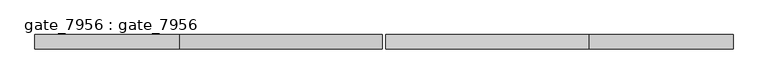
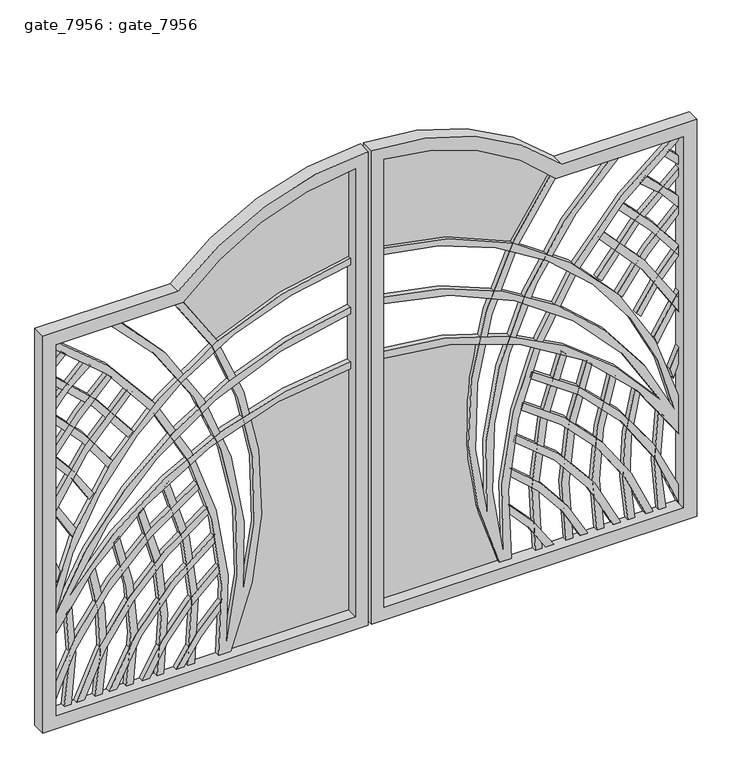
"""IFC4 building model written with IfcOpenShell, lengths in millimetres: proxy geometry, gate_7956 : gate_7956."""

from ifc_helpers import new_model, si_unit, point, frame, frame_2d, origin, place, context, project, spatial, polyline, circle_curve, trimmed, segment, composite_curve, outline, extrude, source, transform, mapped, element, save


def gate_7956_gate_7956_6bc30956(model_context):
    return source(origin(), model_context, "Body", "SweptSolid", [
        extrude(outline(composite_curve([segment(polyline([(1574.8, -714.375), (1574.8, -1222.375), (0.0, -1222.375), (0.0, 0.0), (1879.3736556, 0.0)]), True, "CONTINUOUS"), segment(trimmed(circle_curve(frame_2d((881.859553, 3.175)), 997.5191555), [point((1879.3736556, 0.0))], [point((1574.8, -714.375))], False, "CARTESIAN"), True, "CONTINUOUS")], self_intersect=False), holes=[composite_curve([segment(polyline([(1827.2147875, -47.625), (50.8, -47.625), (50.8, -1171.575), (1524.0, -1171.575), (1524.0, -692.4777911)]), True, "CONTINUOUS"), segment(trimmed(circle_curve(frame_2d((881.859553, 3.175)), 946.7191555), [point((1524.0, -692.4777911))], [point((1827.2147875, -47.625))], True, "CARTESIAN"), True, "CONTINUOUS")], self_intersect=False)]), frame((0.0, -50.8, 0.0), z_axis=(0.0, 1.0, 0.0), x_axis=(0.0, 0.0, 1.0)), (0.0, 0.0, 1.0), 50.8),
        extrude(outline(composite_curve([segment(trimmed(circle_curve(frame_2d((188.1193765, 65.6258097)), 1270.1981582), [point((1453.2587424, -47.625))], [point((475.7606767, -1171.575))], False, "CARTESIAN"), True, "CONTINUOUS"), segment(polyline([(475.7606767, -1171.575), (325.438753, -1171.575)]), True, "CONTINUOUS"), segment(trimmed(circle_curve(frame_2d((-306.470048, -9.2092819)), 1323.0278891), [point((325.438753, -1171.575))], [point((1016.0, -47.625))], True, "CARTESIAN"), True, "CONTINUOUS"), segment(polyline([(1016.0, -47.625), (1042.85139, -47.625)]), True, "CONTINUOUS"), segment(trimmed(circle_curve(frame_2d((-321.9912288, -1.7370637)), 1365.6138095), [point((1042.85139, -47.625))], [point((487.9033995, -1101.269586))], False, "CARTESIAN"), True, "CONTINUOUS"), segment(trimmed(circle_curve(frame_2d((-94.5667128, 101.7568292)), 1336.6166195), [point((487.9033995, -1101.269586))], [point((1233.6761327, -47.625))], True, "CARTESIAN"), True, "CONTINUOUS"), segment(polyline([(1233.6761327, -47.625), (1259.2332506, -47.625)]), True, "CONTINUOUS"), segment(trimmed(circle_curve(frame_2d((-94.5667128, 101.7568292)), 1362.0166195), [point((1259.2332506, -47.625))], [point((428.8390935, -1155.6753295))], False, "CARTESIAN"), True, "CONTINUOUS"), segment(trimmed(circle_curve(frame_2d((188.1193765, 65.6258097)), 1244.7981582), [point((428.8390935, -1155.6753295))], [point((1427.7550927, -47.625))], True, "CARTESIAN"), True, "CONTINUOUS"), segment(polyline([(1427.7550927, -47.625), (1453.2587424, -47.625)]), True, "CONTINUOUS")], self_intersect=False)), frame((0.0, -19.05, 0.0), z_axis=(0.0, 1.0, 0.0), x_axis=(0.0, 0.0, 1.0)), (0.0, 0.0, 1.0), 19.05),
        extrude(outline(composite_curve([segment(trimmed(circle_curve(frame_2d((625.1927136, -1831.8247988)), 1451.1947292), [point((50.8, -499.1436094))], [point((1524.0, -692.4777911))], False, "CARTESIAN"), True, "CONTINUOUS"), segment(polyline([(1524.0, -692.4777911), (1524.0, -717.8616311), (1508.2761961, -712.4096154)]), True, "CONTINUOUS"), segment(trimmed(circle_curve(frame_2d((625.2005352, -1831.8604357)), 1425.8305516), [point((1508.2761961, -712.4096154))], [point((270.5135839, -450.849962))], True, "CARTESIAN"), True, "CONTINUOUS"), segment(trimmed(circle_curve(frame_2d((428.9211986, -1911.4736244)), 1469.1883662), [point((270.5135839, -450.849962))], [point((1524.0, -932.0263955))], False, "CARTESIAN"), True, "CONTINUOUS"), segment(polyline([(1524.0, -932.0263955), (1524.0, -970.5462776)]), True, "CONTINUOUS"), segment(trimmed(circle_curve(frame_2d((434.6192112, -1905.6521568)), 1435.6787622), [point((1524.0, -970.5462776))], [point((79.5169904, -514.5820935))], True, "CARTESIAN"), True, "CONTINUOUS"), segment(trimmed(circle_curve(frame_2d((251.9754674, -2051.8469137)), 1546.9082241), [point((79.5169904, -514.5820935))], [point((1524.0, -1171.575))], False, "CARTESIAN"), True, "CONTINUOUS"), segment(polyline([(1524.0, -1171.575), (1492.986601, -1171.575)]), True, "CONTINUOUS"), segment(trimmed(circle_curve(frame_2d((251.9754674, -2051.8469137)), 1521.5082241), [point((1492.986601, -1171.575))], [point((50.8, -543.6971508))], True, "CARTESIAN"), True, "CONTINUOUS"), segment(polyline([(50.8, -543.6971508), (50.8, -499.1436094)]), True, "CONTINUOUS")], self_intersect=False)), frame((0.0, -19.05, 0.0), z_axis=(0.0, 1.0, 0.0), x_axis=(0.0, 0.0, 1.0)), (0.0, 0.0, 1.0), 19.05),
        extrude(outline(composite_curve([segment(trimmed(circle_curve(frame_2d((-321.9912288, -1.7370636)), 1251.3138095), [point((766.023996, -619.8059275))], [point((122.1545272, -1171.575))], False, "CARTESIAN"), True, "CONTINUOUS"), segment(polyline([(122.1545272, -1171.575), (50.8, -1171.575)]), True, "CONTINUOUS"), segment(trimmed(circle_curve(frame_2d((-329.3476454, 3.2021804)), 1234.7524675), [point((50.8, -1171.575))], [point((741.6413557, -611.2864))], True, "CARTESIAN"), True, "CONTINUOUS"), segment(polyline([(741.6413557, -611.2864), (766.023996, -619.8059275)]), True, "CONTINUOUS")], self_intersect=False)), frame((0.0, -19.05, 0.0), z_axis=(0.0, 1.0, 0.0), x_axis=(0.0, 0.0, 1.0)), (0.0, 0.0, 1.0), 19.05),
        extrude(outline(composite_curve([segment(trimmed(circle_curve(frame_2d((-321.9912288, -1.7370637)), 1137.0138095), [point((654.3216834, -584.5007383))], [point((50.8, -1075.9005069))], False, "CARTESIAN"), True, "CONTINUOUS"), segment(polyline([(50.8, -1075.9005069), (50.8, -1048.9772277)]), True, "CONTINUOUS"), segment(trimmed(circle_curve(frame_2d((-321.9912288, -1.7370637)), 1111.6138095), [point((50.8, -1048.9772277))], [point((628.7552213, -577.7287729))], True, "CARTESIAN"), True, "CONTINUOUS"), segment(polyline([(628.7552213, -577.7287729), (654.3216834, -584.5007383)]), True, "CONTINUOUS")], self_intersect=False)), frame((0.0, -19.05, 0.0), z_axis=(0.0, 1.0, 0.0), x_axis=(0.0, 0.0, 1.0)), (0.0, 0.0, 1.0), 19.05),
        extrude(outline(composite_curve([segment(trimmed(circle_curve(frame_2d((-321.9912288, -1.7370637)), 1022.7138095), [point((536.7182406, -557.2202617))], [point((50.8, -954.0869132))], False, "CARTESIAN"), True, "CONTINUOUS"), segment(polyline([(50.8, -954.0869132), (50.8, -926.7568118)]), True, "CONTINUOUS"), segment(trimmed(circle_curve(frame_2d((-321.9912288, -1.7370637)), 997.3138095), [point((50.8, -926.7568118))], [point((510.8571668, -550.3702604))], True, "CARTESIAN"), True, "CONTINUOUS"), segment(polyline([(510.8571668, -550.3702604), (536.7182406, -557.2202617)]), True, "CONTINUOUS")], self_intersect=False)), frame((0.0, -19.05, 0.0), z_axis=(0.0, 1.0, 0.0), x_axis=(0.0, 0.0, 1.0)), (0.0, 0.0, 1.0), 19.05),
        extrude(outline(composite_curve([segment(trimmed(circle_curve(frame_2d((-321.9912288, -1.7370637)), 908.4138095), [point((410.7722159, -538.6480277))], [point((50.8, -830.134522))], False, "CARTESIAN"), True, "CONTINUOUS"), segment(polyline([(50.8, -830.134522), (50.8, -802.1994847)]), True, "CONTINUOUS"), segment(trimmed(circle_curve(frame_2d((-321.9912288, -1.7370637)), 883.0138095), [point((50.8, -802.1994847))], [point((379.0365912, -538.6480277))], True, "CARTESIAN"), True, "CONTINUOUS"), segment(polyline([(379.0365912, -538.6480277), (410.7722159, -538.6480277)]), True, "CONTINUOUS")], self_intersect=False)), frame((0.0, -19.05, 0.0), z_axis=(0.0, 1.0, 0.0), x_axis=(0.0, 0.0, 1.0)), (0.0, 0.0, 1.0), 19.05),
        extrude(outline(composite_curve([segment(trimmed(circle_curve(frame_2d((-321.9912288, -1.7370637)), 794.1138095), [point((270.5266887, -530.4517881))], [point((50.8, -702.9099683))], False, "CARTESIAN"), True, "CONTINUOUS"), segment(polyline([(50.8, -702.9099683), (50.8, -674.0075603)]), True, "CONTINUOUS"), segment(trimmed(circle_curve(frame_2d((-321.9912288, -1.7370637)), 768.7138095), [point((50.8, -674.0075603))], [point((236.0245963, -530.4517881))], True, "CARTESIAN"), True, "CONTINUOUS"), segment(polyline([(236.0245963, -530.4517881), (270.5266887, -530.4517881)]), True, "CONTINUOUS")], self_intersect=False)), frame((0.0, -19.05, 0.0), z_axis=(0.0, 1.0, 0.0), x_axis=(0.0, 0.0, 1.0)), (0.0, 0.0, 1.0), 19.05),
        extrude(outline(composite_curve([segment(polyline([(1210.9602193, -867.4506933), (1228.939295, -885.429769)]), True, "CONTINUOUS"), segment(trimmed(circle_curve(frame_2d((188.1193765, 65.6258097)), 1409.8981582), [point((1228.939295, -885.429769))], [point((864.245824, -1171.575))], False, "CARTESIAN"), True, "CONTINUOUS"), segment(polyline([(864.245824, -1171.575), (809.5445985, -1171.575)]), True, "CONTINUOUS"), segment(trimmed(circle_curve(frame_2d((188.1193765, 65.6258097)), 1384.4981582), [point((809.5445985, -1171.575))], [point((1210.9602193, -867.4506933))], True, "CARTESIAN"), True, "CONTINUOUS")], self_intersect=False)), frame((0.0, -19.05, 0.0), z_axis=(0.0, 1.0, 0.0), x_axis=(0.0, 0.0, 1.0)), (0.0, 0.0, 1.0), 19.05),
        extrude(outline(composite_curve([segment(polyline([(1295.7670706, -944.0833092), (1313.7464656, -962.0627043)]), True, "CONTINUOUS"), segment(trimmed(circle_curve(frame_2d((298.9547736, -40.580869)), 1370.7410225), [point((1313.7464656, -962.0627043))], [point((1073.4115036, -1171.575))], False, "CARTESIAN"), True, "CONTINUOUS"), segment(polyline([(1073.4115036, -1171.575), (1034.1276953, -1171.575)]), True, "CONTINUOUS"), segment(trimmed(circle_curve(frame_2d((188.1193765, 65.6258097)), 1498.7981582), [point((1034.1276953, -1171.575))], [point((1295.7670706, -944.0833092))], True, "CARTESIAN"), True, "CONTINUOUS")], self_intersect=False)), frame((0.0, -19.05, 0.0), z_axis=(0.0, 1.0, 0.0), x_axis=(0.0, 0.0, 1.0)), (0.0, 0.0, 1.0), 19.05),
        extrude(outline(composite_curve([segment(polyline([(1371.3808408, -1023.8325474), (1393.8084123, -1046.2601189)]), True, "CONTINUOUS"), segment(trimmed(circle_curve(frame_2d((157.0059526, 65.2274597)), 1662.854462), [point((1393.8084123, -1046.2601189))], [point((1268.4935312, -1171.575))], False, "CARTESIAN"), True, "CONTINUOUS"), segment(polyline([(1268.4935312, -1171.575), (1223.2134903, -1171.575)]), True, "CONTINUOUS"), segment(trimmed(circle_curve(frame_2d((881.0604584, -680.2699964)), 598.7063586), [point((1223.2134903, -1171.575))], [point((1371.3808408, -1023.8325474))], True, "CARTESIAN"), True, "CONTINUOUS")], self_intersect=False)), frame((0.0, -19.05, 0.0), z_axis=(0.0, 1.0, 0.0), x_axis=(0.0, 0.0, 1.0)), (0.0, 0.0, 1.0), 19.05),
        extrude(outline(composite_curve([segment(polyline([(1448.1437026, -1116.942791), (1466.2607278, -1135.0598162)]), True, "CONTINUOUS"), segment(trimmed(circle_curve(frame_2d((2369.5144168, -2074.828689)), 1303.469509), [point((1466.2607278, -1135.0598162))], [point((1429.745544, -1171.575))], True, "CARTESIAN"), True, "CONTINUOUS"), segment(polyline([(1429.745544, -1171.575), (1393.6228205, -1171.575)]), True, "CONTINUOUS"), segment(trimmed(circle_curve(frame_2d((2581.8039176, -2302.8138821)), 1640.5717686), [point((1393.6228205, -1171.575))], [point((1448.1437026, -1116.942791))], False, "CARTESIAN"), True, "CONTINUOUS")], self_intersect=False)), frame((0.0, -19.05, 0.0), z_axis=(0.0, 1.0, 0.0), x_axis=(0.0, 0.0, 1.0)), (0.0, 0.0, 1.0), 19.05),
        extrude(outline(composite_curve([segment(polyline([(50.8, -1123.3836365), (50.8, -1096.2682984)]), True, "CONTINUOUS"), segment(trimmed(circle_curve(frame_2d((249.227799, -2294.693819)), 1214.741668), [point((50.8, -1096.2682984))], [point((439.2593722, -1094.9082877))], False, "CARTESIAN"), True, "CONTINUOUS"), segment(polyline([(439.2593722, -1094.9082877), (417.7529701, -1116.4146899)]), True, "CONTINUOUS"), segment(trimmed(circle_curve(frame_2d((251.9754674, -2051.8469137)), 950.0082241), [point((417.7529701, -1116.4146899))], [point((50.8, -1123.3836365))], True, "CARTESIAN"), True, "CONTINUOUS")], self_intersect=False)), frame((0.0, -19.05, 0.0), z_axis=(0.0, 1.0, 0.0), x_axis=(0.0, 0.0, 1.0)), (0.0, 0.0, 1.0), 19.05),
        extrude(outline(composite_curve([segment(polyline([(50.8, -1006.7247069), (50.8, -980.869582)]), True, "CONTINUOUS"), segment(trimmed(circle_curve(frame_2d((251.9754674, -2051.8469137)), 1089.7082241), [point((50.8, -980.869582))], [point((559.4182819, -1006.4078053))], False, "CARTESIAN"), True, "CONTINUOUS"), segment(polyline([(559.4182819, -1006.4078053), (538.8861292, -1026.939958)]), True, "CONTINUOUS"), segment(trimmed(circle_curve(frame_2d((251.9754674, -2051.8469137)), 1064.3082241), [point((538.8861292, -1026.939958))], [point((50.8, -1006.7247069))], True, "CARTESIAN"), True, "CONTINUOUS")], self_intersect=False)), frame((0.0, -19.05, 0.0), z_axis=(0.0, 1.0, 0.0), x_axis=(0.0, 0.0, 1.0)), (0.0, 0.0, 1.0), 19.05),
        extrude(outline(composite_curve([segment(polyline([(50.8, -890.30598), (50.8, -864.7646777)]), True, "CONTINUOUS"), segment(trimmed(circle_curve(frame_2d((251.9754674, -2051.8469137)), 1204.0082241), [point((50.8, -864.7646777))], [point((656.0575932, -917.6716895))], False, "CARTESIAN"), True, "CONTINUOUS"), segment(polyline([(656.0575932, -917.6716895), (636.1282841, -937.6009986)]), True, "CONTINUOUS"), segment(trimmed(circle_curve(frame_2d((249.671635, -2074.7397377)), 1201.0134277), [point((636.1282841, -937.6009986))], [point((50.8, -890.30598))], True, "CARTESIAN"), True, "CONTINUOUS")], self_intersect=False)), frame((0.0, -19.05, 0.0), z_axis=(0.0, 1.0, 0.0), x_axis=(0.0, 0.0, 1.0)), (0.0, 0.0, 1.0), 19.05),
        extrude(outline(composite_curve([segment(polyline([(50.8, -774.6859578), (50.8, -748.9789216)]), True, "CONTINUOUS"), segment(trimmed(circle_curve(frame_2d((251.9754674, -2051.8469137)), 1318.3082241), [point((50.8, -748.9789216))], [point((737.9350335, -826.3756274))], False, "CARTESIAN"), True, "CONTINUOUS"), segment(polyline([(737.9350335, -826.3756274), (718.3335001, -845.9771607)]), True, "CONTINUOUS"), segment(trimmed(circle_curve(frame_2d((251.9754674, -2051.8469137)), 1292.9082241), [point((718.3335001, -845.9771607))], [point((50.8, -774.6859578))], True, "CARTESIAN"), True, "CONTINUOUS")], self_intersect=False)), frame((0.0, -19.05, 0.0), z_axis=(0.0, 1.0, 0.0), x_axis=(0.0, 0.0, 1.0)), (0.0, 0.0, 1.0), 19.05),
        extrude(outline(composite_curve([segment(polyline([(50.8, -659.0930168), (50.8, -633.4341547)]), True, "CONTINUOUS"), segment(trimmed(circle_curve(frame_2d((251.9754674, -2051.8469137)), 1432.6082241), [point((50.8, -633.4341547))], [point((808.380048, -731.7028813))], False, "CARTESIAN"), True, "CONTINUOUS"), segment(polyline([(808.380048, -731.7028813), (788.9599222, -751.1230071)]), True, "CONTINUOUS"), segment(trimmed(circle_curve(frame_2d((251.9754674, -2051.8469137)), 1407.2082241), [point((788.9599222, -751.1230071))], [point((50.8, -659.0930168))], True, "CARTESIAN"), True, "CONTINUOUS")], self_intersect=False)), frame((0.0, -19.05, 0.0), z_axis=(0.0, 1.0, 0.0), x_axis=(0.0, 0.0, 1.0)), (0.0, 0.0, 1.0), 19.05),
        extrude(outline(polyline([(553.3842288, -1150.9205103), (593.450224, -1138.1641492), (672.1451492, -1171.575), (609.2386529, -1171.575), (553.3842288, -1150.9205103)])), frame((0.0, -19.05, 0.0), z_axis=(0.0, 1.0, 0.0), x_axis=(0.0, 0.0, 1.0)), (0.0, 0.0, 1.0), 19.05),
        extrude(outline(composite_curve([segment(trimmed(circle_curve(frame_2d((251.9754673, -2051.8469137)), 1064.3082241), [point((850.2006371, -1171.575))], [point((711.3700205, -1091.7903318))], True, "CARTESIAN"), True, "CONTINUOUS"), segment(polyline([(711.3700205, -1091.7903318), (740.9012216, -1077.980588)]), True, "CONTINUOUS"), segment(trimmed(circle_curve(frame_2d((251.9754674, -2051.8469137)), 1089.7082241), [point((740.9012216, -1077.980588))], [point((894.3035545, -1171.575))], False, "CARTESIAN"), True, "CONTINUOUS"), segment(polyline([(894.3035545, -1171.575), (850.2006371, -1171.575)]), True, "CONTINUOUS")], self_intersect=False)), frame((0.0, -19.05, 0.0), z_axis=(0.0, 1.0, 0.0), x_axis=(0.0, 0.0, 1.0)), (0.0, 0.0, 1.0), 19.05),
        extrude(outline(composite_curve([segment(trimmed(circle_curve(frame_2d((436.5150762, -1780.3292563)), 853.0665783), [point((1034.1276953, -1171.575))], [point((842.2813497, -1029.9451424))], True, "CARTESIAN"), True, "CONTINUOUS"), segment(polyline([(842.2813497, -1029.9451424), (859.7363544, -1012.4901377)]), True, "CONTINUOUS"), segment(trimmed(circle_curve(frame_2d((251.9754673, -2051.8469137)), 1204.0082241), [point((859.7363544, -1012.4901377))], [point((1073.4115036, -1171.575))], False, "CARTESIAN"), True, "CONTINUOUS"), segment(polyline([(1073.4115036, -1171.575), (1034.1276953, -1171.575)]), True, "CONTINUOUS")], self_intersect=False)), frame((0.0, -19.05, 0.0), z_axis=(0.0, 1.0, 0.0), x_axis=(0.0, 0.0, 1.0)), (0.0, 0.0, 1.0), 19.05),
        extrude(outline(composite_curve([segment(polyline([(943.9740273, -959.7161207), (962.3717805, -941.3183675)]), True, "CONTINUOUS"), segment(trimmed(circle_curve(frame_2d((251.9754673, -2051.8469138)), 1318.3082242), [point((962.3717805, -941.3183675))], [point((1233.3306179, -1171.575))], False, "CARTESIAN"), True, "CONTINUOUS"), segment(polyline([(1233.3306179, -1171.575), (1198.9353576, -1171.575)]), True, "CONTINUOUS"), segment(trimmed(circle_curve(frame_2d((251.9754673, -2051.8469138)), 1292.9082241), [point((1198.9353576, -1171.575))], [point((943.9740273, -959.7161207))], True, "CARTESIAN"), True, "CONTINUOUS")], self_intersect=False)), frame((0.0, -19.05, 0.0), z_axis=(0.0, 1.0, 0.0), x_axis=(0.0, 0.0, 1.0)), (0.0, 0.0, 1.0), 19.05),
        extrude(outline(composite_curve([segment(polyline([(1035.0267606, -882.6310833), (1053.3289179, -864.3289261)]), True, "CONTINUOUS"), segment(trimmed(circle_curve(frame_2d((251.9754673, -2051.8469137)), 1432.6082241), [point((1053.3289179, -864.3289261))], [point((1382.2354736, -1171.575))], False, "CARTESIAN"), True, "CONTINUOUS"), segment(polyline([(1382.2354736, -1171.575), (1349.8626855, -1171.575)]), True, "CONTINUOUS"), segment(trimmed(circle_curve(frame_2d((251.9754674, -2051.8469137)), 1407.2082241), [point((1349.8626855, -1171.575))], [point((1035.0267606, -882.6310833))], True, "CARTESIAN"), True, "CONTINUOUS")], self_intersect=False)), frame((0.0, -19.05, 0.0), z_axis=(0.0, 1.0, 0.0), x_axis=(0.0, 0.0, 1.0)), (0.0, 0.0, 1.0), 19.05),
        extrude(outline(composite_curve([segment(trimmed(circle_curve(frame_2d((881.859553, 3.175)), 946.7191555), [point((1827.2147875, -47.625))], [point((1524.0, -692.4777911))], False, "CARTESIAN"), True, "CONTINUOUS"), segment(trimmed(circle_curve(frame_2d((625.1927137, -1831.8247988)), 1451.1947292), [point((1524.0, -692.4777911))], [point((1300.6036994, -547.3847876))], True, "CARTESIAN"), True, "CONTINUOUS"), segment(trimmed(circle_curve(frame_2d((188.1193765, 65.6258097)), 1270.1981582), [point((1300.6036994, -547.3847876))], [point((1453.2587424, -47.625))], True, "CARTESIAN"), True, "CONTINUOUS"), segment(polyline([(1453.2587424, -47.625), (1827.2147875, -47.625)]), True, "CONTINUOUS")], self_intersect=False)), frame((0.0, -6.35, 0.0), z_axis=(0.0, 1.0, 0.0), x_axis=(0.0, 0.0, 1.0)), (0.0, 0.0, 1.0), 6.35),
        extrude(outline(composite_curve([segment(trimmed(circle_curve(frame_2d((-306.470048, -9.2092819)), 1323.0278891), [point((1016.0, -47.625))], [point((951.8602911, -417.8748577))], False, "CARTESIAN"), True, "CONTINUOUS"), segment(trimmed(circle_curve(frame_2d((625.1927136, -1831.8247988)), 1451.1947292), [point((951.8602911, -417.8748577))], [point((50.8, -499.1436094))], True, "CARTESIAN"), True, "CONTINUOUS"), segment(polyline([(50.8, -499.1436094), (50.8, -47.625), (1016.0, -47.625)]), True, "CONTINUOUS")], self_intersect=False)), frame((0.0, -6.35, 0.0), z_axis=(0.0, 1.0, 0.0), x_axis=(0.0, 0.0, 1.0)), (0.0, 0.0, 1.0), 6.35),
        extrude(outline(composite_curve([segment(trimmed(circle_curve(frame_2d((881.859553, 9.525)), 997.5191555), [point((1574.8, 727.075))], [point((1879.3736556, 12.7))], False, "CARTESIAN"), True, "CONTINUOUS"), segment(polyline([(1879.3736556, 12.7), (0.0, 12.7), (0.0, 1235.075), (1574.8, 1235.075), (1574.8, 727.075)]), True, "CONTINUOUS")], self_intersect=False), holes=[composite_curve([segment(trimmed(circle_curve(frame_2d((881.859553, 9.525)), 946.7191555), [point((1827.2147875, 60.325))], [point((1524.0, 705.1777911))], True, "CARTESIAN"), True, "CONTINUOUS"), segment(polyline([(1524.0, 705.1777911), (1524.0, 1184.275), (50.8, 1184.275), (50.8, 60.325), (1827.2147875, 60.325)]), True, "CONTINUOUS")], self_intersect=False)]), frame((0.0, -50.8, 0.0), z_axis=(0.0, 1.0, 0.0), x_axis=(0.0, 0.0, 1.0)), (0.0, 0.0, 1.0), 50.8),
        extrude(outline(composite_curve([segment(polyline([(1453.2587424, 60.325), (1427.7550927, 60.325)]), True, "CONTINUOUS"), segment(trimmed(circle_curve(frame_2d((188.1193765, -52.9258097)), 1244.7981582), [point((1427.7550927, 60.325))], [point((428.8390935, 1168.3753295))], True, "CARTESIAN"), True, "CONTINUOUS"), segment(trimmed(circle_curve(frame_2d((-94.5667128, -89.0568292)), 1362.0166195), [point((428.8390935, 1168.3753295))], [point((1259.2332506, 60.325))], False, "CARTESIAN"), True, "CONTINUOUS"), segment(polyline([(1259.2332506, 60.325), (1233.6761327, 60.325)]), True, "CONTINUOUS"), segment(trimmed(circle_curve(frame_2d((-94.5667128, -89.0568292)), 1336.6166195), [point((1233.6761327, 60.325))], [point((487.9033995, 1113.969586))], True, "CARTESIAN"), True, "CONTINUOUS"), segment(trimmed(circle_curve(frame_2d((-321.9912288, 14.4370637)), 1365.6138095), [point((487.9033995, 1113.969586))], [point((1042.85139, 60.325))], False, "CARTESIAN"), True, "CONTINUOUS"), segment(polyline([(1042.85139, 60.325), (1016.0, 60.325)]), True, "CONTINUOUS"), segment(trimmed(circle_curve(frame_2d((-306.470048, 21.9092819)), 1323.0278891), [point((1016.0, 60.325))], [point((325.438753, 1184.275))], True, "CARTESIAN"), True, "CONTINUOUS"), segment(polyline([(325.438753, 1184.275), (475.7606767, 1184.275)]), True, "CONTINUOUS"), segment(trimmed(circle_curve(frame_2d((188.1193765, -52.9258097)), 1270.1981582), [point((475.7606767, 1184.275))], [point((1453.2587424, 60.325))], False, "CARTESIAN"), True, "CONTINUOUS")], self_intersect=False)), frame((0.0, -19.05, 0.0), z_axis=(0.0, 1.0, 0.0), x_axis=(0.0, 0.0, 1.0)), (0.0, 0.0, 1.0), 19.05),
        extrude(outline(composite_curve([segment(polyline([(50.8, 511.8436094), (50.8, 556.3971508)]), True, "CONTINUOUS"), segment(trimmed(circle_curve(frame_2d((251.9754674, 2064.5469137)), 1521.5082241), [point((50.8, 556.3971508))], [point((1492.986601, 1184.275))], True, "CARTESIAN"), True, "CONTINUOUS"), segment(polyline([(1492.986601, 1184.275), (1524.0, 1184.275)]), True, "CONTINUOUS"), segment(trimmed(circle_curve(frame_2d((251.9754674, 2064.5469137)), 1546.9082241), [point((1524.0, 1184.275))], [point((79.5169904, 527.2820935))], False, "CARTESIAN"), True, "CONTINUOUS"), segment(trimmed(circle_curve(frame_2d((434.6192112, 1918.3521568)), 1435.6787622), [point((79.5169904, 527.2820935))], [point((1524.0, 983.2462776))], True, "CARTESIAN"), True, "CONTINUOUS"), segment(polyline([(1524.0, 983.2462776), (1524.0, 944.7263955)]), True, "CONTINUOUS"), segment(trimmed(circle_curve(frame_2d((428.9211986, 1924.1736244)), 1469.1883662), [point((1524.0, 944.7263955))], [point((270.5135839, 463.549962))], False, "CARTESIAN"), True, "CONTINUOUS"), segment(trimmed(circle_curve(frame_2d((625.2005352, 1844.5604357)), 1425.8305516), [point((270.5135839, 463.549962))], [point((1508.2761961, 725.1096154))], True, "CARTESIAN"), True, "CONTINUOUS"), segment(polyline([(1508.2761961, 725.1096154), (1524.0, 730.5616311), (1524.0, 705.1777911)]), True, "CONTINUOUS"), segment(trimmed(circle_curve(frame_2d((625.1927136, 1844.5247988)), 1451.1947292), [point((1524.0, 705.1777911))], [point((50.8, 511.8436094))], False, "CARTESIAN"), True, "CONTINUOUS")], self_intersect=False)), frame((0.0, -19.05, 0.0), z_axis=(0.0, 1.0, 0.0), x_axis=(0.0, 0.0, 1.0)), (0.0, 0.0, 1.0), 19.05),
        extrude(outline(composite_curve([segment(polyline([(766.023996, 632.5059275), (741.6413557, 623.9864)]), True, "CONTINUOUS"), segment(trimmed(circle_curve(frame_2d((-329.3476454, 9.4978196)), 1234.7524675), [point((741.6413557, 623.9864))], [point((50.8, 1184.275))], True, "CARTESIAN"), True, "CONTINUOUS"), segment(polyline([(50.8, 1184.275), (122.1545272, 1184.275)]), True, "CONTINUOUS"), segment(trimmed(circle_curve(frame_2d((-321.9912288, 14.4370636)), 1251.3138095), [point((122.1545272, 1184.275))], [point((766.023996, 632.5059275))], False, "CARTESIAN"), True, "CONTINUOUS")], self_intersect=False)), frame((0.0, -19.05, 0.0), z_axis=(0.0, 1.0, 0.0), x_axis=(0.0, 0.0, 1.0)), (0.0, 0.0, 1.0), 19.05),
        extrude(outline(composite_curve([segment(polyline([(654.3216834, 597.2007383), (628.7552213, 590.4287729)]), True, "CONTINUOUS"), segment(trimmed(circle_curve(frame_2d((-321.9912288, 14.4370637)), 1111.6138095), [point((628.7552213, 590.4287729))], [point((50.8, 1061.6772277))], True, "CARTESIAN"), True, "CONTINUOUS"), segment(polyline([(50.8, 1061.6772277), (50.8, 1088.6005069)]), True, "CONTINUOUS"), segment(trimmed(circle_curve(frame_2d((-321.9912288, 14.4370637)), 1137.0138095), [point((50.8, 1088.6005069))], [point((654.3216834, 597.2007383))], False, "CARTESIAN"), True, "CONTINUOUS")], self_intersect=False)), frame((0.0, -19.05, 0.0), z_axis=(0.0, 1.0, 0.0), x_axis=(0.0, 0.0, 1.0)), (0.0, 0.0, 1.0), 19.05),
        extrude(outline(composite_curve([segment(polyline([(536.7182406, 569.9202617), (510.8571668, 563.0702604)]), True, "CONTINUOUS"), segment(trimmed(circle_curve(frame_2d((-321.9912288, 14.4370637)), 997.3138095), [point((510.8571668, 563.0702604))], [point((50.8, 939.4568118))], True, "CARTESIAN"), True, "CONTINUOUS"), segment(polyline([(50.8, 939.4568118), (50.8, 966.7869132)]), True, "CONTINUOUS"), segment(trimmed(circle_curve(frame_2d((-321.9912288, 14.4370637)), 1022.7138095), [point((50.8, 966.7869132))], [point((536.7182406, 569.9202617))], False, "CARTESIAN"), True, "CONTINUOUS")], self_intersect=False)), frame((0.0, -19.05, 0.0), z_axis=(0.0, 1.0, 0.0), x_axis=(0.0, 0.0, 1.0)), (0.0, 0.0, 1.0), 19.05),
        extrude(outline(composite_curve([segment(polyline([(410.7722159, 551.3480277), (379.0365912, 551.3480277)]), True, "CONTINUOUS"), segment(trimmed(circle_curve(frame_2d((-321.9912288, 14.4370637)), 883.0138095), [point((379.0365912, 551.3480277))], [point((50.8, 814.8994847))], True, "CARTESIAN"), True, "CONTINUOUS"), segment(polyline([(50.8, 814.8994847), (50.8, 842.834522)]), True, "CONTINUOUS"), segment(trimmed(circle_curve(frame_2d((-321.9912288, 14.4370637)), 908.4138095), [point((50.8, 842.834522))], [point((410.7722159, 551.3480277))], False, "CARTESIAN"), True, "CONTINUOUS")], self_intersect=False)), frame((0.0, -19.05, 0.0), z_axis=(0.0, 1.0, 0.0), x_axis=(0.0, 0.0, 1.0)), (0.0, 0.0, 1.0), 19.05),
        extrude(outline(composite_curve([segment(polyline([(270.5266887, 543.1517881), (236.0245963, 543.1517881)]), True, "CONTINUOUS"), segment(trimmed(circle_curve(frame_2d((-321.9912288, 14.4370637)), 768.7138095), [point((236.0245963, 543.1517881))], [point((50.8, 686.7075603))], True, "CARTESIAN"), True, "CONTINUOUS"), segment(polyline([(50.8, 686.7075603), (50.8, 715.6099683)]), True, "CONTINUOUS"), segment(trimmed(circle_curve(frame_2d((-321.9912288, 14.4370637)), 794.1138095), [point((50.8, 715.6099683))], [point((270.5266887, 543.1517881))], False, "CARTESIAN"), True, "CONTINUOUS")], self_intersect=False)), frame((0.0, -19.05, 0.0), z_axis=(0.0, 1.0, 0.0), x_axis=(0.0, 0.0, 1.0)), (0.0, 0.0, 1.0), 19.05),
        extrude(outline(composite_curve([segment(trimmed(circle_curve(frame_2d((188.1193765, -52.9258097)), 1384.4981582), [point((1210.9602193, 880.1506933))], [point((809.5445985, 1184.275))], True, "CARTESIAN"), True, "CONTINUOUS"), segment(polyline([(809.5445985, 1184.275), (864.245824, 1184.275)]), True, "CONTINUOUS"), segment(trimmed(circle_curve(frame_2d((188.1193765, -52.9258097)), 1409.8981582), [point((864.245824, 1184.275))], [point((1228.939295, 898.129769))], False, "CARTESIAN"), True, "CONTINUOUS"), segment(polyline([(1228.939295, 898.129769), (1210.9602193, 880.1506933)]), True, "CONTINUOUS")], self_intersect=False)), frame((0.0, -19.05, 0.0), z_axis=(0.0, 1.0, 0.0), x_axis=(0.0, 0.0, 1.0)), (0.0, 0.0, 1.0), 19.05),
        extrude(outline(composite_curve([segment(trimmed(circle_curve(frame_2d((188.1193765, -52.9258097)), 1498.7981582), [point((1295.7670706, 956.7833092))], [point((1034.1276953, 1184.275))], True, "CARTESIAN"), True, "CONTINUOUS"), segment(polyline([(1034.1276953, 1184.275), (1073.4115036, 1184.275)]), True, "CONTINUOUS"), segment(trimmed(circle_curve(frame_2d((298.9547736, 53.280869)), 1370.7410225), [point((1073.4115036, 1184.275))], [point((1313.7464656, 974.7627043))], False, "CARTESIAN"), True, "CONTINUOUS"), segment(polyline([(1313.7464656, 974.7627043), (1295.7670706, 956.7833092)]), True, "CONTINUOUS")], self_intersect=False)), frame((0.0, -19.05, 0.0), z_axis=(0.0, 1.0, 0.0), x_axis=(0.0, 0.0, 1.0)), (0.0, 0.0, 1.0), 19.05),
        extrude(outline(composite_curve([segment(trimmed(circle_curve(frame_2d((881.0604584, 692.9699964)), 598.7063586), [point((1371.3808408, 1036.5325474))], [point((1223.2134903, 1184.275))], True, "CARTESIAN"), True, "CONTINUOUS"), segment(polyline([(1223.2134903, 1184.275), (1268.4935312, 1184.275)]), True, "CONTINUOUS"), segment(trimmed(circle_curve(frame_2d((157.0059526, -52.5274597)), 1662.854462), [point((1268.4935312, 1184.275))], [point((1393.8084123, 1058.9601189))], False, "CARTESIAN"), True, "CONTINUOUS"), segment(polyline([(1393.8084123, 1058.9601189), (1371.3808408, 1036.5325474)]), True, "CONTINUOUS")], self_intersect=False)), frame((0.0, -19.05, 0.0), z_axis=(0.0, 1.0, 0.0), x_axis=(0.0, 0.0, 1.0)), (0.0, 0.0, 1.0), 19.05),
        extrude(outline(composite_curve([segment(trimmed(circle_curve(frame_2d((2581.8039176, 2315.5138821)), 1640.5717686), [point((1448.1437026, 1129.642791))], [point((1393.6228205, 1184.275))], False, "CARTESIAN"), True, "CONTINUOUS"), segment(polyline([(1393.6228205, 1184.275), (1429.745544, 1184.275)]), True, "CONTINUOUS"), segment(trimmed(circle_curve(frame_2d((2369.5144168, 2087.528689)), 1303.469509), [point((1429.745544, 1184.275))], [point((1466.2607278, 1147.7598162))], True, "CARTESIAN"), True, "CONTINUOUS"), segment(polyline([(1466.2607278, 1147.7598162), (1448.1437026, 1129.642791)]), True, "CONTINUOUS")], self_intersect=False)), frame((0.0, -19.05, 0.0), z_axis=(0.0, 1.0, 0.0), x_axis=(0.0, 0.0, 1.0)), (0.0, 0.0, 1.0), 19.05),
        extrude(outline(composite_curve([segment(trimmed(circle_curve(frame_2d((251.9754674, 2064.5469137)), 950.0082241), [point((50.8, 1136.0836365))], [point((417.7529701, 1129.1146899))], True, "CARTESIAN"), True, "CONTINUOUS"), segment(polyline([(417.7529701, 1129.1146899), (439.2593722, 1107.6082877)]), True, "CONTINUOUS"), segment(trimmed(circle_curve(frame_2d((249.227799, 2307.393819)), 1214.741668), [point((439.2593722, 1107.6082877))], [point((50.8, 1108.9682984))], False, "CARTESIAN"), True, "CONTINUOUS"), segment(polyline([(50.8, 1108.9682984), (50.8, 1136.0836365)]), True, "CONTINUOUS")], self_intersect=False)), frame((0.0, -19.05, 0.0), z_axis=(0.0, 1.0, 0.0), x_axis=(0.0, 0.0, 1.0)), (0.0, 0.0, 1.0), 19.05),
        extrude(outline(composite_curve([segment(trimmed(circle_curve(frame_2d((251.9754674, 2064.5469137)), 1064.3082241), [point((50.8, 1019.4247069))], [point((538.8861292, 1039.639958))], True, "CARTESIAN"), True, "CONTINUOUS"), segment(polyline([(538.8861292, 1039.639958), (559.4182819, 1019.1078053)]), True, "CONTINUOUS"), segment(trimmed(circle_curve(frame_2d((251.9754674, 2064.5469137)), 1089.7082241), [point((559.4182819, 1019.1078053))], [point((50.8, 993.569582))], False, "CARTESIAN"), True, "CONTINUOUS"), segment(polyline([(50.8, 993.569582), (50.8, 1019.4247069)]), True, "CONTINUOUS")], self_intersect=False)), frame((0.0, -19.05, 0.0), z_axis=(0.0, 1.0, 0.0), x_axis=(0.0, 0.0, 1.0)), (0.0, 0.0, 1.0), 19.05),
        extrude(outline(composite_curve([segment(trimmed(circle_curve(frame_2d((249.671635, 2087.4397377)), 1201.0134277), [point((50.8, 903.00598))], [point((636.1282841, 950.3009986))], True, "CARTESIAN"), True, "CONTINUOUS"), segment(polyline([(636.1282841, 950.3009986), (656.0575932, 930.3716895)]), True, "CONTINUOUS"), segment(trimmed(circle_curve(frame_2d((251.9754674, 2064.5469137)), 1204.0082241), [point((656.0575932, 930.3716895))], [point((50.8, 877.4646777))], False, "CARTESIAN"), True, "CONTINUOUS"), segment(polyline([(50.8, 877.4646777), (50.8, 903.00598)]), True, "CONTINUOUS")], self_intersect=False)), frame((0.0, -19.05, 0.0), z_axis=(0.0, 1.0, 0.0), x_axis=(0.0, 0.0, 1.0)), (0.0, 0.0, 1.0), 19.05),
        extrude(outline(composite_curve([segment(trimmed(circle_curve(frame_2d((251.9754674, 2064.5469137)), 1292.9082241), [point((50.8, 787.3859578))], [point((718.3335001, 858.6771607))], True, "CARTESIAN"), True, "CONTINUOUS"), segment(polyline([(718.3335001, 858.6771607), (737.9350335, 839.0756274)]), True, "CONTINUOUS"), segment(trimmed(circle_curve(frame_2d((251.9754674, 2064.5469137)), 1318.3082241), [point((737.9350335, 839.0756274))], [point((50.8, 761.6789216))], False, "CARTESIAN"), True, "CONTINUOUS"), segment(polyline([(50.8, 761.6789216), (50.8, 787.3859578)]), True, "CONTINUOUS")], self_intersect=False)), frame((0.0, -19.05, 0.0), z_axis=(0.0, 1.0, 0.0), x_axis=(0.0, 0.0, 1.0)), (0.0, 0.0, 1.0), 19.05),
        extrude(outline(composite_curve([segment(trimmed(circle_curve(frame_2d((251.9754674, 2064.5469137)), 1407.2082241), [point((50.8, 671.7930168))], [point((788.9599222, 763.8230071))], True, "CARTESIAN"), True, "CONTINUOUS"), segment(polyline([(788.9599222, 763.8230071), (808.380048, 744.4028813)]), True, "CONTINUOUS"), segment(trimmed(circle_curve(frame_2d((251.9754674, 2064.5469137)), 1432.6082241), [point((808.380048, 744.4028813))], [point((50.8, 646.1341547))], False, "CARTESIAN"), True, "CONTINUOUS"), segment(polyline([(50.8, 646.1341547), (50.8, 671.7930168)]), True, "CONTINUOUS")], self_intersect=False)), frame((0.0, -19.05, 0.0), z_axis=(0.0, 1.0, 0.0), x_axis=(0.0, 0.0, 1.0)), (0.0, 0.0, 1.0), 19.05),
        extrude(outline(polyline([(553.3842288, 1163.6205103), (609.2386529, 1184.275), (672.1451492, 1184.275), (593.450224, 1150.8641492), (553.3842288, 1163.6205103)])), frame((0.0, -19.05, 0.0), z_axis=(0.0, 1.0, 0.0), x_axis=(0.0, 0.0, 1.0)), (0.0, 0.0, 1.0), 19.05),
        extrude(outline(composite_curve([segment(polyline([(850.2006371, 1184.275), (894.3035545, 1184.275)]), True, "CONTINUOUS"), segment(trimmed(circle_curve(frame_2d((251.9754674, 2064.5469137)), 1089.7082241), [point((894.3035545, 1184.275))], [point((740.9012216, 1090.680588))], False, "CARTESIAN"), True, "CONTINUOUS"), segment(polyline([(740.9012216, 1090.680588), (711.3700205, 1104.4903318)]), True, "CONTINUOUS"), segment(trimmed(circle_curve(frame_2d((251.9754673, 2064.5469137)), 1064.3082241), [point((711.3700205, 1104.4903318))], [point((850.2006371, 1184.275))], True, "CARTESIAN"), True, "CONTINUOUS")], self_intersect=False)), frame((0.0, -19.05, 0.0), z_axis=(0.0, 1.0, 0.0), x_axis=(0.0, 0.0, 1.0)), (0.0, 0.0, 1.0), 19.05),
        extrude(outline(composite_curve([segment(polyline([(1034.1276953, 1184.275), (1073.4115036, 1184.275)]), True, "CONTINUOUS"), segment(trimmed(circle_curve(frame_2d((251.9754673, 2064.5469137)), 1204.0082241), [point((1073.4115036, 1184.275))], [point((859.7363544, 1025.1901377))], False, "CARTESIAN"), True, "CONTINUOUS"), segment(polyline([(859.7363544, 1025.1901377), (842.2813497, 1042.6451424)]), True, "CONTINUOUS"), segment(trimmed(circle_curve(frame_2d((436.5150762, 1793.0292563)), 853.0665783), [point((842.2813497, 1042.6451424))], [point((1034.1276953, 1184.275))], True, "CARTESIAN"), True, "CONTINUOUS")], self_intersect=False)), frame((0.0, -19.05, 0.0), z_axis=(0.0, 1.0, 0.0), x_axis=(0.0, 0.0, 1.0)), (0.0, 0.0, 1.0), 19.05),
        extrude(outline(composite_curve([segment(trimmed(circle_curve(frame_2d((251.9754673, 2064.5469138)), 1292.9082241), [point((943.9740273, 972.4161207))], [point((1198.9353576, 1184.275))], True, "CARTESIAN"), True, "CONTINUOUS"), segment(polyline([(1198.9353576, 1184.275), (1233.3306179, 1184.275)]), True, "CONTINUOUS"), segment(trimmed(circle_curve(frame_2d((251.9754673, 2064.5469138)), 1318.3082242), [point((1233.3306179, 1184.275))], [point((962.3717805, 954.0183675))], False, "CARTESIAN"), True, "CONTINUOUS"), segment(polyline([(962.3717805, 954.0183675), (943.9740273, 972.4161207)]), True, "CONTINUOUS")], self_intersect=False)), frame((0.0, -19.05, 0.0), z_axis=(0.0, 1.0, 0.0), x_axis=(0.0, 0.0, 1.0)), (0.0, 0.0, 1.0), 19.05),
        extrude(outline(composite_curve([segment(trimmed(circle_curve(frame_2d((251.9754674, 2064.5469137)), 1407.2082241), [point((1035.0267606, 895.3310833))], [point((1349.8626855, 1184.275))], True, "CARTESIAN"), True, "CONTINUOUS"), segment(polyline([(1349.8626855, 1184.275), (1382.2354736, 1184.275)]), True, "CONTINUOUS"), segment(trimmed(circle_curve(frame_2d((251.9754673, 2064.5469137)), 1432.6082241), [point((1382.2354736, 1184.275))], [point((1053.3289179, 877.0289261))], False, "CARTESIAN"), True, "CONTINUOUS"), segment(polyline([(1053.3289179, 877.0289261), (1035.0267606, 895.3310833)]), True, "CONTINUOUS")], self_intersect=False)), frame((0.0, -19.05, 0.0), z_axis=(0.0, 1.0, 0.0), x_axis=(0.0, 0.0, 1.0)), (0.0, 0.0, 1.0), 19.05),
        extrude(outline(composite_curve([segment(polyline([(1827.2147875, 60.325), (1453.2587424, 60.325)]), True, "CONTINUOUS"), segment(trimmed(circle_curve(frame_2d((188.1193765, -52.9258097)), 1270.1981582), [point((1453.2587424, 60.325))], [point((1300.6036994, 560.0847876))], True, "CARTESIAN"), True, "CONTINUOUS"), segment(trimmed(circle_curve(frame_2d((625.1927137, 1844.5247988)), 1451.1947292), [point((1300.6036994, 560.0847876))], [point((1524.0, 705.1777911))], True, "CARTESIAN"), True, "CONTINUOUS"), segment(trimmed(circle_curve(frame_2d((881.859553, 9.525)), 946.7191555), [point((1524.0, 705.1777911))], [point((1827.2147875, 60.325))], False, "CARTESIAN"), True, "CONTINUOUS")], self_intersect=False)), frame((0.0, -6.35, 0.0), z_axis=(0.0, 1.0, 0.0), x_axis=(0.0, 0.0, 1.0)), (0.0, 0.0, 1.0), 6.35),
        extrude(outline(composite_curve([segment(polyline([(1016.0, 60.325), (50.8, 60.325), (50.8, 511.8436094)]), True, "CONTINUOUS"), segment(trimmed(circle_curve(frame_2d((625.1927136, 1844.5247988)), 1451.1947292), [point((50.8, 511.8436094))], [point((951.8602911, 430.5748577))], True, "CARTESIAN"), True, "CONTINUOUS"), segment(trimmed(circle_curve(frame_2d((-306.470048, 21.9092819)), 1323.0278891), [point((951.8602911, 430.5748577))], [point((1016.0, 60.325))], False, "CARTESIAN"), True, "CONTINUOUS")], self_intersect=False)), frame((0.0, -6.35, 0.0), z_axis=(0.0, 1.0, 0.0), x_axis=(0.0, 0.0, 1.0)), (0.0, 0.0, 1.0), 6.35),
    ])


if __name__ == "__main__":
    model = new_model("IFC4")
    model_context = context("Model", 3, world=origin())
    ifc_project = project(units=[si_unit("LENGTHUNIT", "METRE", prefix="MILLI")], contexts=[model_context])
    site = spatial("IfcSite", under=ifc_project)
    building = spatial("IfcBuilding", under=site)
    placement = place(None, origin())
    gate_7956_gate_7956_shape = gate_7956_gate_7956_6bc30956(model_context)
    element("IfcBuildingElementProxy", 1, Name="gate_7956 : gate_7956", ObjectType="gate_7956 : gate_7956", at=placement, inside=building, context=model_context, shape_type="MappedRepresentation", body=[
        mapped(gate_7956_gate_7956_shape, transform((0.0, 0.0, 0.0), x_axis=(1.0, 0.0, 0.0), y_axis=(0.0, 1.0, 0.0), z_axis=(0.0, 0.0, 1.0))),
    ])
    save(model, "model.ifc")

# Revit data of these elements
# Type "gate_7956 : gate_7956"
#   m.s. sheet = none
#   2" x2" pipe = none
#   1"x1"pipe = none
#   Default Elevation = 0
